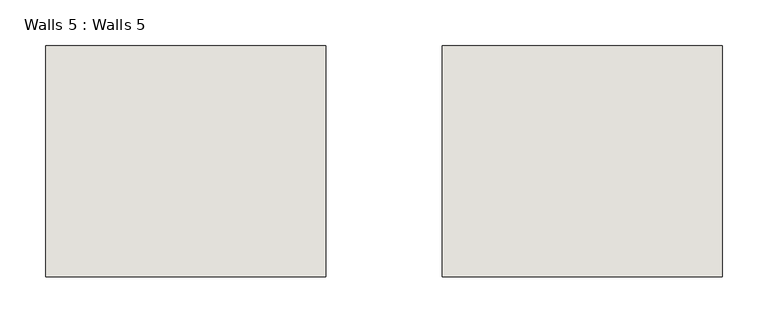
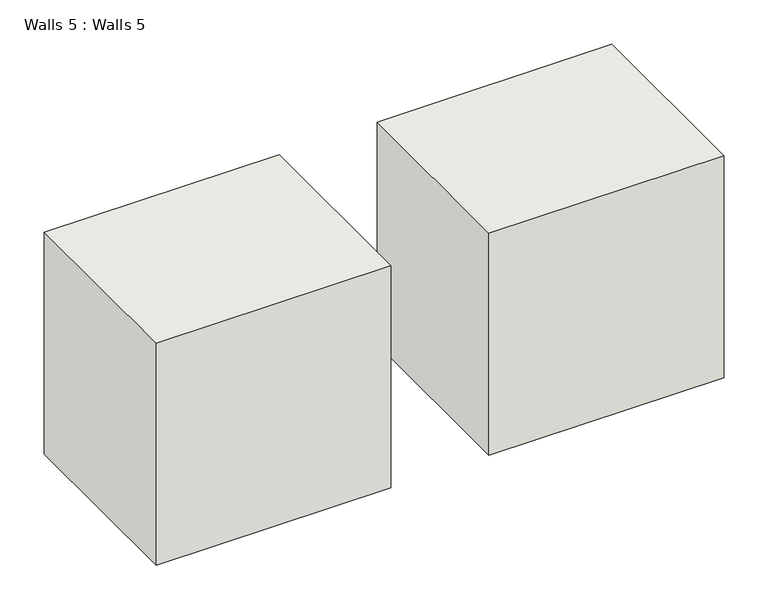
"""IFC4 building model written with IfcOpenShell, lengths in millimetres: wall geometry, Walls 5 : Walls 5."""

from ifc_helpers import new_model, si_unit, frame, origin, place, context, project, spatial, polyline, outline, extrude, source, transform, mapped, element, save


def walls_5_walls_5_3445876a(model_context):
    return source(origin(), model_context, "Body", "SweptSolid", [
        extrude(outline(polyline([(-7506.9283887, -4082.4116874), (-7811.7283887, -4082.4116874), (-7811.7283887, -3830.9620523), (-7506.9283887, -3830.9620523), (-7506.9283887, -4082.4116874)])), frame((0.0, 0.0, 4304.231532), z_axis=(0.0, 0.0, 1.0), x_axis=(1.0, 0.0, 0.0)), (0.0, 0.0, 1.0), 304.8),
        extrude(outline(polyline([(-7075.1283887, -4082.4116874), (-7379.9283887, -4082.4116874), (-7379.9283887, -3830.9620523), (-7075.1283887, -3830.9620523), (-7075.1283887, -4082.4116874)])), frame((0.0, 0.0, 4304.231532), z_axis=(0.0, 0.0, 1.0), x_axis=(1.0, 0.0, 0.0)), (0.0, 0.0, 1.0), 304.8),
    ])


if __name__ == "__main__":
    model = new_model("IFC4")
    model_context = context("Model", 3, world=origin())
    ifc_project = project(units=[si_unit("LENGTHUNIT", "METRE", prefix="MILLI")], contexts=[model_context])
    site = spatial("IfcSite", under=ifc_project)
    building = spatial("IfcBuilding", under=site)
    placement = place(None, origin())
    walls_5_walls_5_shape = walls_5_walls_5_3445876a(model_context)
    element("IfcWall", 1, ObjectType="Walls 5 : Walls 5", at=placement, inside=building, context=model_context, shape_type="MappedRepresentation", body=[
        mapped(walls_5_walls_5_shape, transform((0.0, 0.0, 0.0), x_axis=(1.0, 0.0, 0.0), y_axis=(0.0, 1.0, 0.0), z_axis=(0.0, 0.0, 1.0))),
    ])
    save(model, "model.ifc")

# Revit data of these elements
# Element 1 (IfcWall, "Walls 5 : Walls 5")
#   Materials on its faces: "Default Wall"
# Materials
#   "Default Wall": colour RGB 128 128 128, transparency 0
